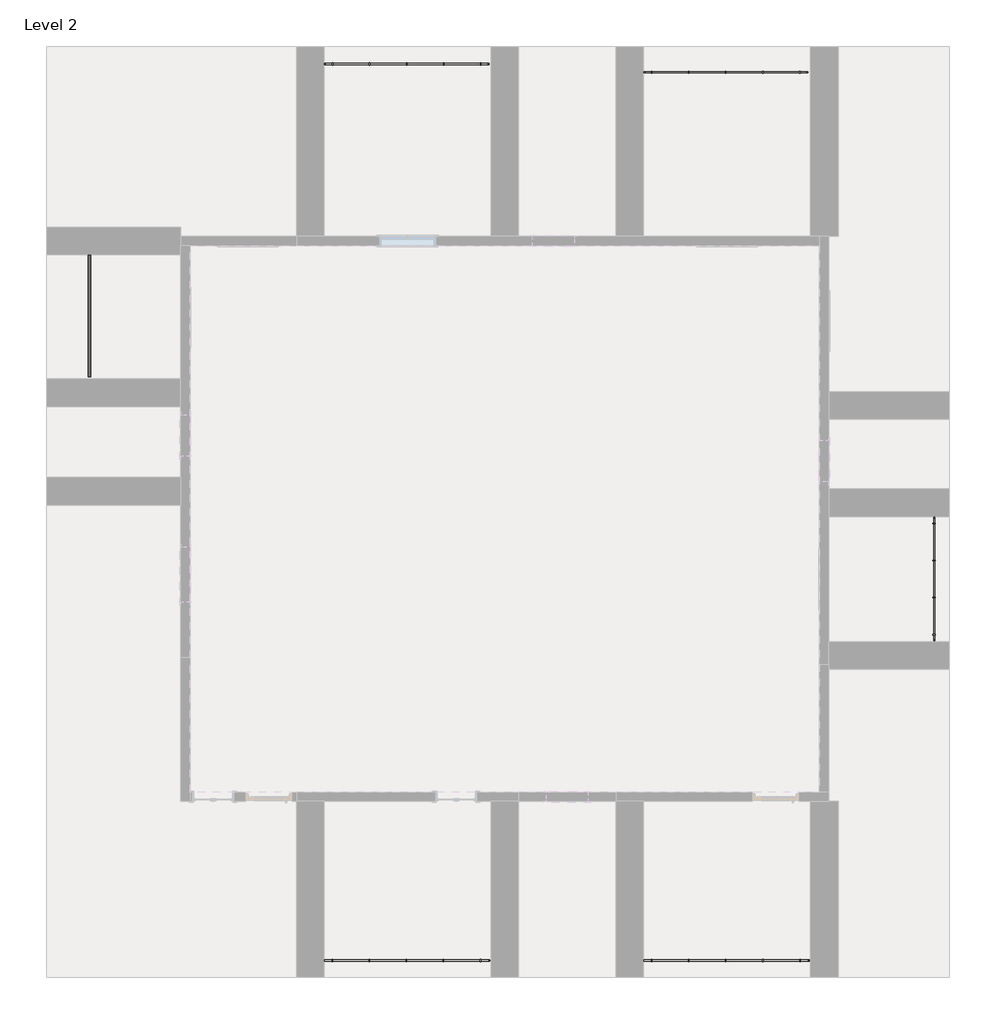
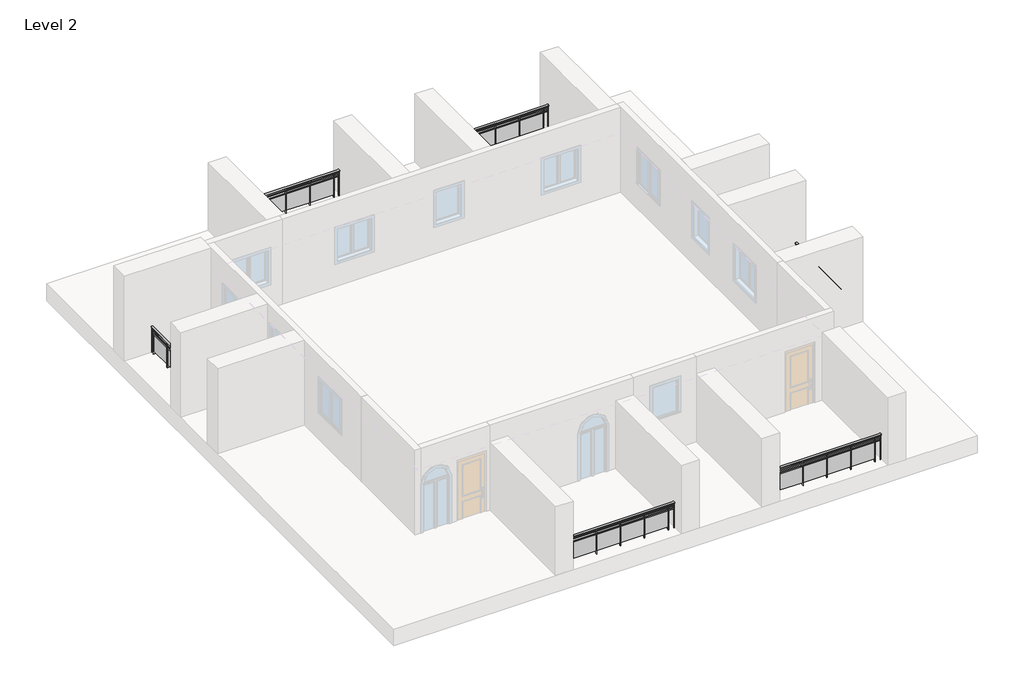
# One storey, part 2 of 2: 6 railings.
"""IFC4 building model written with IfcOpenShell, lengths in millimetres."""

from ifc_helpers import new_model, si_unit, point, frame, origin, place, context, project, spatial, polyline, ellipse_curve, trimmed, outline, extrude, element, save
from ifc_brep_helpers import plane_surface, extruded_surface, advanced_brep

model = new_model("IFC4")

# Units and contexts
model_context = context("Model", 3, world=origin())
ifc_project = project(units=[si_unit("LENGTHUNIT", "METRE", prefix="MILLI")], contexts=[model_context])

# Site, building, storey
site = spatial("IfcSite", under=ifc_project)
building = spatial("IfcBuilding", under=site)
storey = spatial("IfcBuildingStorey", under=building, Name="Level 2", Elevation=3048.0)

# Railings
placement = place(None, origin())
element("IfcRailing", 1, ObjectType="Glass Panel - Bottom Fill", at=placement, inside=storey, context=model_context, shape_type="SolidModel", body=[
    advanced_brep(
    [(-9258.4937431, -9324.2034265, 4267.2), (-9258.4937431, -9400.4034265, 4267.2), (-5600.8937431, -9324.2034265, 4267.2), (-5600.8937431, -9400.4034265, 4267.2)],
    [
        (0, 1, ellipse_curve(frame((-9258.4937431, -9362.3034265, 4267.2), z_axis=(-1.0, 0.0, 0.0), x_axis=(0.0, -1.0, 0.0)), 38.1, 28.575)),
        (1, 0, ellipse_curve(frame((-9258.4937431, -9362.3034265, 4267.2), z_axis=(-1.0, 0.0, 0.0), x_axis=(0.0, -1.0, 0.0)), 38.1, 28.575)),
        (2, 3, ellipse_curve(frame((-5600.8937431, -9362.3034265, 4267.2), z_axis=(1.0, 0.0, 0.0), x_axis=(0.0, -1.0, 0.0)), 38.1, 28.575)),
        (3, 2, ellipse_curve(frame((-5600.8937431, -9362.3034265, 4267.2), z_axis=(1.0, 0.0, 0.0), x_axis=(0.0, -1.0, 0.0)), 38.1, 28.575)),
        (0, 2),
        (3, 1),
    ],
    [
        plane_surface(frame((-9258.4937431, -9362.3034265, 4267.2), z_axis=(-1.0, 0.0, 0.0), x_axis=(0.0, 1.0, 0.0))),
        plane_surface(frame((-5600.8937431, -9362.3034265, 4267.2), z_axis=(1.0, 0.0, 0.0), x_axis=(0.0, 1.0, 0.0))),
        extruded_surface(trimmed(ellipse_curve(frame((-5600.8937431, -9362.3034265, 4267.2), z_axis=(-1.0, 0.0, 0.0), x_axis=(0.0, -1.0, 0.0)), 38.1, 28.575), [point((-5600.8937431, -9324.2034265, 4267.2))], [point((-5600.8937431, -9400.4034265, 4267.2))], True, "CARTESIAN"), (-3657.5999999999995, 0.0, 0.0), 3657.5999999999995),
        extruded_surface(trimmed(ellipse_curve(frame((-5600.8937431, -9362.3034265, 4267.2), z_axis=(-1.0, 0.0, 0.0), x_axis=(0.0, -1.0, 0.0)), 38.1, 28.575), [point((-5600.8937431, -9400.4034265, 4267.2))], [point((-5600.8937431, -9324.2034265, 4267.2))], True, "CARTESIAN"), (-3657.5999999999995, 0.0, 0.0), 3657.5999999999995),
    ],
    [
        (0, [[1, 2]]),
        (1, [[3, 4]]),
        (2, [[-1, 5, -4, 6]]),
        (3, [[-2, -6, -3, -5]]),
    ],
),
    extrude(outline(polyline([(-9258.4937431, -9375.0034265), (-9258.4937431, -9349.6034265), (-5600.8937431, -9349.6034265), (-5600.8937431, -9375.0034265), (-9258.4937431, -9375.0034265)])), frame((0.0, 0.0, 4152.9), z_axis=(0.0, 0.0, 1.0), x_axis=(1.0, 0.0, 0.0)), (0.0, 0.0, 1.0), 25.4),
    extrude(outline(polyline([(-9258.4937431, -9375.0034265), (-9258.4937431, -9349.6034265), (-5600.8937431, -9349.6034265), (-5600.8937431, -9375.0034265), (-9258.4937431, -9375.0034265)])), frame((0.0, 0.0, 4051.3), z_axis=(0.0, 0.0, 1.0), x_axis=(1.0, 0.0, 0.0)), (0.0, 0.0, 1.0), 25.4),
    extrude(outline(polyline([(-5810.4437431, -9387.7034265), (-5810.4437431, -9336.9034265), (-5797.7437431, -9336.9034265), (-5797.7437431, -9387.7034265), (-5810.4437431, -9387.7034265)])), frame((0.0, 0.0, 3352.8), z_axis=(0.0, 0.0, 1.0), x_axis=(1.0, 0.0, 0.0)), (0.0, 0.0, 1.0), 885.6788223),
    extrude(outline(polyline([(-6616.8937431, -9355.7682695), (-5804.0937431, -9355.7682695), (-5804.0937431, -9362.1182695), (-6616.8937431, -9362.1182695), (-6616.8937431, -9355.7682695)])), frame((0.0, 0.0, 3454.4), z_axis=(0.0, 0.0, 1.0), x_axis=(1.0, 0.0, 0.0)), (0.0, 0.0, 1.0), 596.9),
    extrude(outline(polyline([(-6623.2437431, -9387.7034265), (-6623.2437431, -9336.9034265), (-6610.5437431, -9336.9034265), (-6610.5437431, -9387.7034265), (-6623.2437431, -9387.7034265)])), frame((0.0, 0.0, 3352.8), z_axis=(0.0, 0.0, 1.0), x_axis=(1.0, 0.0, 0.0)), (0.0, 0.0, 1.0), 885.6788223),
    extrude(outline(polyline([(-7429.6937431, -9355.7682695), (-6616.8937431, -9355.7682695), (-6616.8937431, -9362.1182695), (-7429.6937431, -9362.1182695), (-7429.6937431, -9355.7682695)])), frame((0.0, 0.0, 3454.4), z_axis=(0.0, 0.0, 1.0), x_axis=(1.0, 0.0, 0.0)), (0.0, 0.0, 1.0), 596.9),
    extrude(outline(polyline([(-7436.0437431, -9387.7034265), (-7436.0437431, -9336.9034265), (-7423.3437431, -9336.9034265), (-7423.3437431, -9387.7034265), (-7436.0437431, -9387.7034265)])), frame((0.0, 0.0, 3352.8), z_axis=(0.0, 0.0, 1.0), x_axis=(1.0, 0.0, 0.0)), (0.0, 0.0, 1.0), 885.6788223),
    extrude(outline(polyline([(-8242.4937431, -9355.7682695), (-7429.6937431, -9355.7682695), (-7429.6937431, -9362.1182695), (-8242.4937431, -9362.1182695), (-8242.4937431, -9355.7682695)])), frame((0.0, 0.0, 3454.4), z_axis=(0.0, 0.0, 1.0), x_axis=(1.0, 0.0, 0.0)), (0.0, 0.0, 1.0), 596.9),
    extrude(outline(polyline([(-8248.8437431, -9387.7034265), (-8248.8437431, -9336.9034265), (-8236.1437431, -9336.9034265), (-8236.1437431, -9387.7034265), (-8248.8437431, -9387.7034265)])), frame((0.0, 0.0, 3352.8), z_axis=(0.0, 0.0, 1.0), x_axis=(1.0, 0.0, 0.0)), (0.0, 0.0, 1.0), 885.6788223),
    extrude(outline(polyline([(-9055.2937431, -9355.7682695), (-8242.4937431, -9355.7682695), (-8242.4937431, -9362.1182695), (-9055.2937431, -9362.1182695), (-9055.2937431, -9355.7682695)])), frame((0.0, 0.0, 3454.4), z_axis=(0.0, 0.0, 1.0), x_axis=(1.0, 0.0, 0.0)), (0.0, 0.0, 1.0), 596.9),
    extrude(outline(polyline([(-9061.6437431, -9387.7034265), (-9061.6437431, -9336.9034265), (-9048.9437431, -9336.9034265), (-9048.9437431, -9387.7034265), (-9061.6437431, -9387.7034265)])), frame((0.0, 0.0, 3352.8), z_axis=(0.0, 0.0, 1.0), x_axis=(1.0, 0.0, 0.0)), (0.0, 0.0, 1.0), 885.6788223),
    extrude(outline(polyline([(-5613.5937431, -9371.8284265), (-5613.5937431, -9352.7784265), (-5594.5437431, -9352.7784265), (-5594.5437431, -9371.8284265), (-5613.5937431, -9371.8284265)])), frame((0.0, 0.0, 3352.8), z_axis=(0.0, 0.0, 1.0), x_axis=(1.0, 0.0, 0.0)), (0.0, 0.0, 1.0), 885.6788223),
    extrude(outline(polyline([(-9264.8437431, -9371.8284265), (-9264.8437431, -9352.7784265), (-9245.7937431, -9352.7784265), (-9245.7937431, -9371.8284265), (-9264.8437431, -9371.8284265)])), frame((0.0, 0.0, 3352.8), z_axis=(0.0, 0.0, 1.0), x_axis=(1.0, 0.0, 0.0)), (0.0, 0.0, 1.0), 885.6788223),
])
element("IfcRailing", 2, ObjectType="Glass Panel - Bottom Fill", at=placement, inside=storey, context=model_context, shape_type="SolidModel", body=[
    advanced_brep(
    [(-2248.0325613, -9324.2034265, 4262.1393423), (-2248.0325613, -9400.4034265, 4262.1393423), (1409.5674387, -9324.2034265, 4262.1393423), (1409.5674387, -9400.4034265, 4262.1393423)],
    [
        (0, 1, ellipse_curve(frame((-2248.0325613, -9362.3034265, 4262.1393423), z_axis=(-1.0, 0.0, 0.0), x_axis=(0.0, -1.0, 0.0)), 38.1, 28.575)),
        (1, 0, ellipse_curve(frame((-2248.0325613, -9362.3034265, 4262.1393423), z_axis=(-1.0, 0.0, 0.0), x_axis=(0.0, -1.0, 0.0)), 38.1, 28.575)),
        (2, 3, ellipse_curve(frame((1409.5674387, -9362.3034265, 4262.1393423), z_axis=(1.0, 0.0, 0.0), x_axis=(0.0, -1.0, 0.0)), 38.1, 28.575)),
        (3, 2, ellipse_curve(frame((1409.5674387, -9362.3034265, 4262.1393423), z_axis=(1.0, 0.0, 0.0), x_axis=(0.0, -1.0, 0.0)), 38.1, 28.575)),
        (0, 2),
        (3, 1),
    ],
    [
        plane_surface(frame((-2248.0325613, -9362.3034265, 4262.1393423), z_axis=(-1.0, 0.0, 0.0), x_axis=(0.0, 1.0, 0.0))),
        plane_surface(frame((1409.5674387, -9362.3034265, 4262.1393423), z_axis=(1.0, 0.0, 0.0), x_axis=(0.0, 1.0, 0.0))),
        extruded_surface(trimmed(ellipse_curve(frame((1409.5674387, -9362.3034265, 4262.1393423), z_axis=(-1.0, 0.0, 0.0), x_axis=(0.0, -1.0, 0.0)), 38.1, 28.575), [point((1409.5674387, -9324.2034265, 4262.1393423))], [point((1409.5674387, -9400.4034265, 4262.1393423))], True, "CARTESIAN"), (-3657.6, 0.0, 0.0), 3657.6),
        extruded_surface(trimmed(ellipse_curve(frame((1409.5674387, -9362.3034265, 4262.1393423), z_axis=(-1.0, 0.0, 0.0), x_axis=(0.0, -1.0, 0.0)), 38.1, 28.575), [point((1409.5674387, -9400.4034265, 4262.1393423))], [point((1409.5674387, -9324.2034265, 4262.1393423))], True, "CARTESIAN"), (-3657.6, 0.0, 0.0), 3657.6),
    ],
    [
        (0, [[1, 2]]),
        (1, [[3, 4]]),
        (2, [[-1, 5, -4, 6]]),
        (3, [[-2, -6, -3, -5]]),
    ],
),
    extrude(outline(polyline([(-2248.0325613, -9375.0034265), (-2248.0325613, -9349.6034265), (1409.5674387, -9349.6034265), (1409.5674387, -9375.0034265), (-2248.0325613, -9375.0034265)])), frame((0.0, 0.0, 4147.8393423), z_axis=(0.0, 0.0, 1.0), x_axis=(1.0, 0.0, 0.0)), (0.0, 0.0, 1.0), 25.4),
    extrude(outline(polyline([(-2248.0325613, -9375.0034265), (-2248.0325613, -9349.6034265), (1409.5674387, -9349.6034265), (1409.5674387, -9375.0034265), (-2248.0325613, -9375.0034265)])), frame((0.0, 0.0, 4046.2393423), z_axis=(0.0, 0.0, 1.0), x_axis=(1.0, 0.0, 0.0)), (0.0, 0.0, 1.0), 25.4),
    extrude(outline(polyline([(1200.0174387, -9387.7034265), (1200.0174387, -9336.9034265), (1212.7174387, -9336.9034265), (1212.7174387, -9387.7034265), (1200.0174387, -9387.7034265)])), frame((0.0, 0.0, 3347.7393423), z_axis=(0.0, 0.0, 1.0), x_axis=(1.0, 0.0, 0.0)), (0.0, 0.0, 1.0), 885.6788223),
    extrude(outline(polyline([(393.5674387, -9355.7682695), (1206.3674387, -9355.7682695), (1206.3674387, -9362.1182695), (393.5674387, -9362.1182695), (393.5674387, -9355.7682695)])), frame((0.0, 0.0, 3449.3393423), z_axis=(0.0, 0.0, 1.0), x_axis=(1.0, 0.0, 0.0)), (0.0, 0.0, 1.0), 596.9),
    extrude(outline(polyline([(387.2174387, -9387.7034265), (387.2174387, -9336.9034265), (399.9174387, -9336.9034265), (399.9174387, -9387.7034265), (387.2174387, -9387.7034265)])), frame((0.0, 0.0, 3347.7393423), z_axis=(0.0, 0.0, 1.0), x_axis=(1.0, 0.0, 0.0)), (0.0, 0.0, 1.0), 885.6788223),
    extrude(outline(polyline([(-419.2325613, -9355.7682695), (393.5674387, -9355.7682695), (393.5674387, -9362.1182695), (-419.2325613, -9362.1182695), (-419.2325613, -9355.7682695)])), frame((0.0, 0.0, 3449.3393423), z_axis=(0.0, 0.0, 1.0), x_axis=(1.0, 0.0, 0.0)), (0.0, 0.0, 1.0), 596.9),
    extrude(outline(polyline([(-425.5825613, -9387.7034265), (-425.5825613, -9336.9034265), (-412.8825613, -9336.9034265), (-412.8825613, -9387.7034265), (-425.5825613, -9387.7034265)])), frame((0.0, 0.0, 3347.7393423), z_axis=(0.0, 0.0, 1.0), x_axis=(1.0, 0.0, 0.0)), (0.0, 0.0, 1.0), 885.6788223),
    extrude(outline(polyline([(-1232.0325613, -9355.7682695), (-419.2325613, -9355.7682695), (-419.2325613, -9362.1182695), (-1232.0325613, -9362.1182695), (-1232.0325613, -9355.7682695)])), frame((0.0, 0.0, 3449.3393423), z_axis=(0.0, 0.0, 1.0), x_axis=(1.0, 0.0, 0.0)), (0.0, 0.0, 1.0), 596.9),
    extrude(outline(polyline([(-1238.3825613, -9387.7034265), (-1238.3825613, -9336.9034265), (-1225.6825613, -9336.9034265), (-1225.6825613, -9387.7034265), (-1238.3825613, -9387.7034265)])), frame((0.0, 0.0, 3347.7393423), z_axis=(0.0, 0.0, 1.0), x_axis=(1.0, 0.0, 0.0)), (0.0, 0.0, 1.0), 885.6788223),
    extrude(outline(polyline([(-2044.8325613, -9355.7682695), (-1232.0325613, -9355.7682695), (-1232.0325613, -9362.1182695), (-2044.8325613, -9362.1182695), (-2044.8325613, -9355.7682695)])), frame((0.0, 0.0, 3449.3393423), z_axis=(0.0, 0.0, 1.0), x_axis=(1.0, 0.0, 0.0)), (0.0, 0.0, 1.0), 596.9),
    extrude(outline(polyline([(-2051.1825613, -9387.7034265), (-2051.1825613, -9336.9034265), (-2038.4825613, -9336.9034265), (-2038.4825613, -9387.7034265), (-2051.1825613, -9387.7034265)])), frame((0.0, 0.0, 3347.7393423), z_axis=(0.0, 0.0, 1.0), x_axis=(1.0, 0.0, 0.0)), (0.0, 0.0, 1.0), 885.6788223),
    extrude(outline(polyline([(1396.8674387, -9371.8284265), (1396.8674387, -9352.7784265), (1415.9174387, -9352.7784265), (1415.9174387, -9371.8284265), (1396.8674387, -9371.8284265)])), frame((0.0, 0.0, 3347.7393423), z_axis=(0.0, 0.0, 1.0), x_axis=(1.0, 0.0, 0.0)), (0.0, 0.0, 1.0), 885.6788223),
    extrude(outline(polyline([(-2254.3825613, -9371.8284265), (-2254.3825613, -9352.7784265), (-2235.3325613, -9352.7784265), (-2235.3325613, -9371.8284265), (-2254.3825613, -9371.8284265)])), frame((0.0, 0.0, 3347.7393423), z_axis=(0.0, 0.0, 1.0), x_axis=(1.0, 0.0, 0.0)), (0.0, 0.0, 1.0), 885.6788223),
])
element("IfcRailing", 3, ObjectType="Glass Panel - Bottom Fill", at=placement, inside=storey, context=model_context, shape_type="SolidModel", body=[
    advanced_brep(
    [(-14351.1937431, 6115.813611, 4267.2), (-14427.3937431, 6115.813611, 4267.2), (-14351.1937431, 3448.813611, 4267.2), (-14427.3937431, 3448.813611, 4267.2)],
    [
        (0, 1, ellipse_curve(frame((-14389.2937431, 6115.813611, 4267.2), z_axis=(0.0, 1.0, 0.0), x_axis=(-1.0, 0.0, 0.0)), 38.1, 28.575)),
        (1, 0, ellipse_curve(frame((-14389.2937431, 6115.813611, 4267.2), z_axis=(0.0, 1.0, 0.0), x_axis=(-1.0, 0.0, 0.0)), 38.1, 28.575)),
        (2, 3, ellipse_curve(frame((-14389.2937431, 3448.813611, 4267.2), z_axis=(0.0, -1.0, 0.0), x_axis=(-1.0, 0.0, 0.0)), 38.1, 28.575)),
        (3, 2, ellipse_curve(frame((-14389.2937431, 3448.813611, 4267.2), z_axis=(0.0, -1.0, 0.0), x_axis=(-1.0, 0.0, 0.0)), 38.1, 28.575)),
        (0, 2),
        (3, 1),
    ],
    [
        plane_surface(frame((-14389.2937431, 6115.813611, 4267.2), z_axis=(0.0, 1.0, 0.0), x_axis=(0.0, 0.0, -1.0))),
        plane_surface(frame((-14389.2937431, 3448.813611, 4267.2), z_axis=(0.0, -1.0, 0.0), x_axis=(0.0, 0.0, -1.0))),
        extruded_surface(trimmed(ellipse_curve(frame((-14389.2937431, 3448.813611, 4267.2), z_axis=(0.0, 1.0, 0.0), x_axis=(-1.0, 0.0, 0.0)), 38.1, 28.575), [point((-14351.1937431, 3448.813611, 4267.2))], [point((-14427.3937431, 3448.813611, 4267.2))], True, "CARTESIAN"), (0.0, 2666.9999999999995, 0.0), 2666.9999999999995),
        extruded_surface(trimmed(ellipse_curve(frame((-14389.2937431, 3448.813611, 4267.2), z_axis=(0.0, 1.0, 0.0), x_axis=(-1.0, 0.0, 0.0)), 38.1, 28.575), [point((-14427.3937431, 3448.813611, 4267.2))], [point((-14351.1937431, 3448.813611, 4267.2))], True, "CARTESIAN"), (0.0, 2666.9999999999995, 0.0), 2666.9999999999995),
    ],
    [
        (0, [[1, 2]]),
        (1, [[3, 4]]),
        (2, [[-1, 5, -4, 6]]),
        (3, [[-2, -6, -3, -5]]),
    ],
),
    extrude(outline(polyline([(-14401.9937431, 6115.813611), (-14376.5937431, 6115.813611), (-14376.5937431, 3448.813611), (-14401.9937431, 3448.813611), (-14401.9937431, 6115.813611)])), frame((0.0, 0.0, 4152.9), z_axis=(0.0, 0.0, 1.0), x_axis=(1.0, 0.0, 0.0)), (0.0, 0.0, 1.0), 25.4),
    extrude(outline(polyline([(-14401.9937431, 6115.813611), (-14376.5937431, 6115.813611), (-14376.5937431, 3448.813611), (-14401.9937431, 3448.813611), (-14401.9937431, 6115.813611)])), frame((0.0, 0.0, 4051.3), z_axis=(0.0, 0.0, 1.0), x_axis=(1.0, 0.0, 0.0)), (0.0, 0.0, 1.0), 25.4),
    extrude(outline(polyline([(-14414.6937431, 3569.463611), (-14363.8937431, 3569.463611), (-14363.8937431, 3556.763611), (-14414.6937431, 3556.763611), (-14414.6937431, 3569.463611)])), frame((0.0, 0.0, 3352.8), z_axis=(0.0, 0.0, 1.0), x_axis=(1.0, 0.0, 0.0)), (0.0, 0.0, 1.0), 885.6788223),
    extrude(outline(polyline([(-14382.7585861, 4375.913611), (-14382.7585861, 3563.113611), (-14389.1085861, 3563.113611), (-14389.1085861, 4375.913611), (-14382.7585861, 4375.913611)])), frame((0.0, 0.0, 3454.4), z_axis=(0.0, 0.0, 1.0), x_axis=(1.0, 0.0, 0.0)), (0.0, 0.0, 1.0), 596.9),
    extrude(outline(polyline([(-14414.6937431, 4382.263611), (-14363.8937431, 4382.263611), (-14363.8937431, 4369.563611), (-14414.6937431, 4369.563611), (-14414.6937431, 4382.263611)])), frame((0.0, 0.0, 3352.8), z_axis=(0.0, 0.0, 1.0), x_axis=(1.0, 0.0, 0.0)), (0.0, 0.0, 1.0), 885.6788223),
    extrude(outline(polyline([(-14382.7585861, 5188.713611), (-14382.7585861, 4375.913611), (-14389.1085861, 4375.913611), (-14389.1085861, 5188.713611), (-14382.7585861, 5188.713611)])), frame((0.0, 0.0, 3454.4), z_axis=(0.0, 0.0, 1.0), x_axis=(1.0, 0.0, 0.0)), (0.0, 0.0, 1.0), 596.9),
    extrude(outline(polyline([(-14414.6937431, 5195.063611), (-14363.8937431, 5195.063611), (-14363.8937431, 5182.363611), (-14414.6937431, 5182.363611), (-14414.6937431, 5195.063611)])), frame((0.0, 0.0, 3352.8), z_axis=(0.0, 0.0, 1.0), x_axis=(1.0, 0.0, 0.0)), (0.0, 0.0, 1.0), 885.6788223),
    extrude(outline(polyline([(-14382.7585861, 6001.513611), (-14382.7585861, 5188.713611), (-14389.1085861, 5188.713611), (-14389.1085861, 6001.513611), (-14382.7585861, 6001.513611)])), frame((0.0, 0.0, 3454.4), z_axis=(0.0, 0.0, 1.0), x_axis=(1.0, 0.0, 0.0)), (0.0, 0.0, 1.0), 596.9),
    extrude(outline(polyline([(-14414.6937431, 6007.863611), (-14363.8937431, 6007.863611), (-14363.8937431, 5995.163611), (-14414.6937431, 5995.163611), (-14414.6937431, 6007.863611)])), frame((0.0, 0.0, 3352.8), z_axis=(0.0, 0.0, 1.0), x_axis=(1.0, 0.0, 0.0)), (0.0, 0.0, 1.0), 885.6788223),
    extrude(outline(polyline([(-14398.8187431, 3461.513611), (-14379.7687431, 3461.513611), (-14379.7687431, 3442.463611), (-14398.8187431, 3442.463611), (-14398.8187431, 3461.513611)])), frame((0.0, 0.0, 3352.8), z_axis=(0.0, 0.0, 1.0), x_axis=(1.0, 0.0, 0.0)), (0.0, 0.0, 1.0), 885.6788223),
    extrude(outline(polyline([(-14398.8187431, 6122.163611), (-14379.7687431, 6122.163611), (-14379.7687431, 6103.113611), (-14398.8187431, 6103.113611), (-14398.8187431, 6122.163611)])), frame((0.0, 0.0, 3352.8), z_axis=(0.0, 0.0, 1.0), x_axis=(1.0, 0.0, 0.0)), (0.0, 0.0, 1.0), 885.6788223),
])
element("IfcRailing", 4, ObjectType="Glass Panel - Bottom Fill", at=placement, inside=storey, context=model_context, shape_type="SolidModel", body=[
    advanced_brep(
    [(-9229.0758442, 10344.5205237, 4267.2), (-9229.0758442, 10268.3205237, 4267.2), (-5622.2758442, 10344.5205237, 4267.2), (-5622.2758442, 10268.3205237, 4267.2)],
    [
        (0, 1, ellipse_curve(frame((-9229.0758442, 10306.4205237, 4267.2), z_axis=(-1.0, 0.0, 0.0), x_axis=(0.0, -1.0, 0.0)), 38.1, 28.575)),
        (1, 0, ellipse_curve(frame((-9229.0758442, 10306.4205237, 4267.2), z_axis=(-1.0, 0.0, 0.0), x_axis=(0.0, -1.0, 0.0)), 38.1, 28.575)),
        (2, 3, ellipse_curve(frame((-5622.2758442, 10306.4205237, 4267.2), z_axis=(1.0, 0.0, 0.0), x_axis=(0.0, -1.0, 0.0)), 38.1, 28.575)),
        (3, 2, ellipse_curve(frame((-5622.2758442, 10306.4205237, 4267.2), z_axis=(1.0, 0.0, 0.0), x_axis=(0.0, -1.0, 0.0)), 38.1, 28.575)),
        (0, 2),
        (3, 1),
    ],
    [
        plane_surface(frame((-9229.0758442, 10306.4205237, 4267.2), z_axis=(-1.0, 0.0, 0.0), x_axis=(0.0, 1.0, 0.0))),
        plane_surface(frame((-5622.2758442, 10306.4205237, 4267.2), z_axis=(1.0, 0.0, 0.0), x_axis=(0.0, 1.0, 0.0))),
        extruded_surface(trimmed(ellipse_curve(frame((-5622.2758442, 10306.4205237, 4267.2), z_axis=(-1.0, 0.0, 0.0), x_axis=(0.0, -1.0, 0.0)), 38.1, 28.575), [point((-5622.2758442, 10344.5205237, 4267.2))], [point((-5622.2758442, 10268.3205237, 4267.2))], True, "CARTESIAN"), (-3606.8, 0.0, 0.0), 3606.8),
        extruded_surface(trimmed(ellipse_curve(frame((-5622.2758442, 10306.4205237, 4267.2), z_axis=(-1.0, 0.0, 0.0), x_axis=(0.0, -1.0, 0.0)), 38.1, 28.575), [point((-5622.2758442, 10268.3205237, 4267.2))], [point((-5622.2758442, 10344.5205237, 4267.2))], True, "CARTESIAN"), (-3606.8, 0.0, 0.0), 3606.8),
    ],
    [
        (0, [[1, 2]]),
        (1, [[3, 4]]),
        (2, [[-1, 5, -4, 6]]),
        (3, [[-2, -6, -3, -5]]),
    ],
),
    extrude(outline(polyline([(-9229.0758442, 10293.7205237), (-9229.0758442, 10319.1205237), (-5622.2758442, 10319.1205237), (-5622.2758442, 10293.7205237), (-9229.0758442, 10293.7205237)])), frame((0.0, 0.0, 4152.9), z_axis=(0.0, 0.0, 1.0), x_axis=(1.0, 0.0, 0.0)), (0.0, 0.0, 1.0), 25.4),
    extrude(outline(polyline([(-9229.0758442, 10293.7205237), (-9229.0758442, 10319.1205237), (-5622.2758442, 10319.1205237), (-5622.2758442, 10293.7205237), (-9229.0758442, 10293.7205237)])), frame((0.0, 0.0, 4051.3), z_axis=(0.0, 0.0, 1.0), x_axis=(1.0, 0.0, 0.0)), (0.0, 0.0, 1.0), 25.4),
    extrude(outline(polyline([(-5806.4258442, 10281.0205237), (-5806.4258442, 10331.8205237), (-5793.7258442, 10331.8205237), (-5793.7258442, 10281.0205237), (-5806.4258442, 10281.0205237)])), frame((0.0, 0.0, 3352.8), z_axis=(0.0, 0.0, 1.0), x_axis=(1.0, 0.0, 0.0)), (0.0, 0.0, 1.0), 885.6788223),
    extrude(outline(polyline([(-6612.8758442, 10312.9556807), (-5800.0758442, 10312.9556807), (-5800.0758442, 10306.6056807), (-6612.8758442, 10306.6056807), (-6612.8758442, 10312.9556807)])), frame((0.0, 0.0, 3454.4), z_axis=(0.0, 0.0, 1.0), x_axis=(1.0, 0.0, 0.0)), (0.0, 0.0, 1.0), 596.9),
    extrude(outline(polyline([(-6619.2258442, 10281.0205237), (-6619.2258442, 10331.8205237), (-6606.5258442, 10331.8205237), (-6606.5258442, 10281.0205237), (-6619.2258442, 10281.0205237)])), frame((0.0, 0.0, 3352.8), z_axis=(0.0, 0.0, 1.0), x_axis=(1.0, 0.0, 0.0)), (0.0, 0.0, 1.0), 885.6788223),
    extrude(outline(polyline([(-7425.6758442, 10312.9556807), (-6612.8758442, 10312.9556807), (-6612.8758442, 10306.6056807), (-7425.6758442, 10306.6056807), (-7425.6758442, 10312.9556807)])), frame((0.0, 0.0, 3454.4), z_axis=(0.0, 0.0, 1.0), x_axis=(1.0, 0.0, 0.0)), (0.0, 0.0, 1.0), 596.9),
    extrude(outline(polyline([(-7432.0258442, 10281.0205237), (-7432.0258442, 10331.8205237), (-7419.3258442, 10331.8205237), (-7419.3258442, 10281.0205237), (-7432.0258442, 10281.0205237)])), frame((0.0, 0.0, 3352.8), z_axis=(0.0, 0.0, 1.0), x_axis=(1.0, 0.0, 0.0)), (0.0, 0.0, 1.0), 885.6788223),
    extrude(outline(polyline([(-8238.4758442, 10312.9556807), (-7425.6758442, 10312.9556807), (-7425.6758442, 10306.6056807), (-8238.4758442, 10306.6056807), (-8238.4758442, 10312.9556807)])), frame((0.0, 0.0, 3454.4), z_axis=(0.0, 0.0, 1.0), x_axis=(1.0, 0.0, 0.0)), (0.0, 0.0, 1.0), 596.9),
    extrude(outline(polyline([(-8244.8258442, 10281.0205237), (-8244.8258442, 10331.8205237), (-8232.1258442, 10331.8205237), (-8232.1258442, 10281.0205237), (-8244.8258442, 10281.0205237)])), frame((0.0, 0.0, 3352.8), z_axis=(0.0, 0.0, 1.0), x_axis=(1.0, 0.0, 0.0)), (0.0, 0.0, 1.0), 885.6788223),
    extrude(outline(polyline([(-9051.2758442, 10312.9556807), (-8238.4758442, 10312.9556807), (-8238.4758442, 10306.6056807), (-9051.2758442, 10306.6056807), (-9051.2758442, 10312.9556807)])), frame((0.0, 0.0, 3454.4), z_axis=(0.0, 0.0, 1.0), x_axis=(1.0, 0.0, 0.0)), (0.0, 0.0, 1.0), 596.9),
    extrude(outline(polyline([(-9057.6258442, 10281.0205237), (-9057.6258442, 10331.8205237), (-9044.9258442, 10331.8205237), (-9044.9258442, 10281.0205237), (-9057.6258442, 10281.0205237)])), frame((0.0, 0.0, 3352.8), z_axis=(0.0, 0.0, 1.0), x_axis=(1.0, 0.0, 0.0)), (0.0, 0.0, 1.0), 885.6788223),
    extrude(outline(polyline([(-5634.9758442, 10296.8955237), (-5634.9758442, 10315.9455237), (-5615.9258442, 10315.9455237), (-5615.9258442, 10296.8955237), (-5634.9758442, 10296.8955237)])), frame((0.0, 0.0, 3352.8), z_axis=(0.0, 0.0, 1.0), x_axis=(1.0, 0.0, 0.0)), (0.0, 0.0, 1.0), 885.6788223),
    extrude(outline(polyline([(-9235.4258442, 10296.8955237), (-9235.4258442, 10315.9455237), (-9216.3758442, 10315.9455237), (-9216.3758442, 10296.8955237), (-9235.4258442, 10296.8955237)])), frame((0.0, 0.0, 3352.8), z_axis=(0.0, 0.0, 1.0), x_axis=(1.0, 0.0, 0.0)), (0.0, 0.0, 1.0), 885.6788223),
])
element("IfcRailing", 5, ObjectType="Glass Panel - Bottom Fill", at=placement, inside=storey, context=model_context, shape_type="SolidModel", body=[
    advanced_brep(
    [(-2210.3891352, 10161.3373193, 4267.2), (-2210.3891352, 10085.1373193, 4267.2), (1371.0108648, 10161.3373193, 4267.2), (1371.0108648, 10085.1373193, 4267.2)],
    [
        (0, 1, ellipse_curve(frame((-2210.3891352, 10123.2373193, 4267.2), z_axis=(-1.0, 0.0, 0.0), x_axis=(0.0, -1.0, 0.0)), 38.1, 28.575)),
        (1, 0, ellipse_curve(frame((-2210.3891352, 10123.2373193, 4267.2), z_axis=(-1.0, 0.0, 0.0), x_axis=(0.0, -1.0, 0.0)), 38.1, 28.575)),
        (2, 3, ellipse_curve(frame((1371.0108648, 10123.2373193, 4267.2), z_axis=(1.0, 0.0, 0.0), x_axis=(0.0, -1.0, 0.0)), 38.1, 28.575)),
        (3, 2, ellipse_curve(frame((1371.0108648, 10123.2373193, 4267.2), z_axis=(1.0, 0.0, 0.0), x_axis=(0.0, -1.0, 0.0)), 38.1, 28.575)),
        (0, 2),
        (3, 1),
    ],
    [
        plane_surface(frame((-2210.3891352, 10123.2373193, 4267.2), z_axis=(-1.0, 0.0, 0.0), x_axis=(0.0, 1.0, 0.0))),
        plane_surface(frame((1371.0108648, 10123.2373193, 4267.2), z_axis=(1.0, 0.0, 0.0), x_axis=(0.0, 1.0, 0.0))),
        extruded_surface(trimmed(ellipse_curve(frame((1371.0108648, 10123.2373193, 4267.2), z_axis=(-1.0, 0.0, 0.0), x_axis=(0.0, -1.0, 0.0)), 38.1, 28.575), [point((1371.0108648, 10161.3373193, 4267.2))], [point((1371.0108648, 10085.1373193, 4267.2))], True, "CARTESIAN"), (-3581.4, 0.0, 0.0), 3581.4),
        extruded_surface(trimmed(ellipse_curve(frame((1371.0108648, 10123.2373193, 4267.2), z_axis=(-1.0, 0.0, 0.0), x_axis=(0.0, -1.0, 0.0)), 38.1, 28.575), [point((1371.0108648, 10085.1373193, 4267.2))], [point((1371.0108648, 10161.3373193, 4267.2))], True, "CARTESIAN"), (-3581.4, 0.0, 0.0), 3581.4),
    ],
    [
        (0, [[1, 2]]),
        (1, [[3, 4]]),
        (2, [[-1, 5, -4, 6]]),
        (3, [[-2, -6, -3, -5]]),
    ],
),
    extrude(outline(polyline([(-2210.3891352, 10110.5373193), (-2210.3891352, 10135.9373193), (1371.0108648, 10135.9373193), (1371.0108648, 10110.5373193), (-2210.3891352, 10110.5373193)])), frame((0.0, 0.0, 4152.9), z_axis=(0.0, 0.0, 1.0), x_axis=(1.0, 0.0, 0.0)), (0.0, 0.0, 1.0), 25.4),
    extrude(outline(polyline([(-2210.3891352, 10110.5373193), (-2210.3891352, 10135.9373193), (1371.0108648, 10135.9373193), (1371.0108648, 10110.5373193), (-2210.3891352, 10110.5373193)])), frame((0.0, 0.0, 4051.3), z_axis=(0.0, 0.0, 1.0), x_axis=(1.0, 0.0, 0.0)), (0.0, 0.0, 1.0), 25.4),
    extrude(outline(polyline([(1199.5608648, 10097.8373193), (1199.5608648, 10148.6373193), (1212.2608648, 10148.6373193), (1212.2608648, 10097.8373193), (1199.5608648, 10097.8373193)])), frame((0.0, 0.0, 3352.8), z_axis=(0.0, 0.0, 1.0), x_axis=(1.0, 0.0, 0.0)), (0.0, 0.0, 1.0), 885.6788223),
    extrude(outline(polyline([(393.1108648, 10129.7724763), (1205.9108648, 10129.7724763), (1205.9108648, 10123.4224763), (393.1108648, 10123.4224763), (393.1108648, 10129.7724763)])), frame((0.0, 0.0, 3454.4), z_axis=(0.0, 0.0, 1.0), x_axis=(1.0, 0.0, 0.0)), (0.0, 0.0, 1.0), 596.9),
    extrude(outline(polyline([(386.7608648, 10097.8373193), (386.7608648, 10148.6373193), (399.4608648, 10148.6373193), (399.4608648, 10097.8373193), (386.7608648, 10097.8373193)])), frame((0.0, 0.0, 3352.8), z_axis=(0.0, 0.0, 1.0), x_axis=(1.0, 0.0, 0.0)), (0.0, 0.0, 1.0), 885.6788223),
    extrude(outline(polyline([(-419.6891352, 10129.7724763), (393.1108648, 10129.7724763), (393.1108648, 10123.4224763), (-419.6891352, 10123.4224763), (-419.6891352, 10129.7724763)])), frame((0.0, 0.0, 3454.4), z_axis=(0.0, 0.0, 1.0), x_axis=(1.0, 0.0, 0.0)), (0.0, 0.0, 1.0), 596.9),
    extrude(outline(polyline([(-426.0391352, 10097.8373193), (-426.0391352, 10148.6373193), (-413.3391352, 10148.6373193), (-413.3391352, 10097.8373193), (-426.0391352, 10097.8373193)])), frame((0.0, 0.0, 3352.8), z_axis=(0.0, 0.0, 1.0), x_axis=(1.0, 0.0, 0.0)), (0.0, 0.0, 1.0), 885.6788223),
    extrude(outline(polyline([(-1232.4891352, 10129.7724763), (-419.6891352, 10129.7724763), (-419.6891352, 10123.4224763), (-1232.4891352, 10123.4224763), (-1232.4891352, 10129.7724763)])), frame((0.0, 0.0, 3454.4), z_axis=(0.0, 0.0, 1.0), x_axis=(1.0, 0.0, 0.0)), (0.0, 0.0, 1.0), 596.9),
    extrude(outline(polyline([(-1238.8391352, 10097.8373193), (-1238.8391352, 10148.6373193), (-1226.1391352, 10148.6373193), (-1226.1391352, 10097.8373193), (-1238.8391352, 10097.8373193)])), frame((0.0, 0.0, 3352.8), z_axis=(0.0, 0.0, 1.0), x_axis=(1.0, 0.0, 0.0)), (0.0, 0.0, 1.0), 885.6788223),
    extrude(outline(polyline([(-2045.2891352, 10129.7724763), (-1232.4891352, 10129.7724763), (-1232.4891352, 10123.4224763), (-2045.2891352, 10123.4224763), (-2045.2891352, 10129.7724763)])), frame((0.0, 0.0, 3454.4), z_axis=(0.0, 0.0, 1.0), x_axis=(1.0, 0.0, 0.0)), (0.0, 0.0, 1.0), 596.9),
    extrude(outline(polyline([(-2051.6391352, 10097.8373193), (-2051.6391352, 10148.6373193), (-2038.9391352, 10148.6373193), (-2038.9391352, 10097.8373193), (-2051.6391352, 10097.8373193)])), frame((0.0, 0.0, 3352.8), z_axis=(0.0, 0.0, 1.0), x_axis=(1.0, 0.0, 0.0)), (0.0, 0.0, 1.0), 885.6788223),
    extrude(outline(polyline([(1358.3108648, 10113.7123193), (1358.3108648, 10132.7623193), (1377.3608648, 10132.7623193), (1377.3608648, 10113.7123193), (1358.3108648, 10113.7123193)])), frame((0.0, 0.0, 3352.8), z_axis=(0.0, 0.0, 1.0), x_axis=(1.0, 0.0, 0.0)), (0.0, 0.0, 1.0), 885.6788223),
    extrude(outline(polyline([(-2216.7391352, 10113.7123193), (-2216.7391352, 10132.7623193), (-2197.6891352, 10132.7623193), (-2197.6891352, 10113.7123193), (-2216.7391352, 10113.7123193)])), frame((0.0, 0.0, 3352.8), z_axis=(0.0, 0.0, 1.0), x_axis=(1.0, 0.0, 0.0)), (0.0, 0.0, 1.0), 885.6788223),
])
element("IfcRailing", 6, ObjectType="Glass Panel - Bottom Fill", at=placement, inside=storey, context=model_context, shape_type="SolidModel", body=[
    advanced_brep(
    [(4190.8062569, 350.013611, 4267.2), (4114.6062569, 350.013611, 4267.2), (4190.8062569, -2342.386389, 4267.2), (4114.6062569, -2342.386389, 4267.2)],
    [
        (0, 1, ellipse_curve(frame((4152.7062569, 350.013611, 4267.2), z_axis=(0.0, 1.0, 0.0), x_axis=(-1.0, 0.0, 0.0)), 38.1, 28.575)),
        (1, 0, ellipse_curve(frame((4152.7062569, 350.013611, 4267.2), z_axis=(0.0, 1.0, 0.0), x_axis=(-1.0, 0.0, 0.0)), 38.1, 28.575)),
        (2, 3, ellipse_curve(frame((4152.7062569, -2342.386389, 4267.2), z_axis=(0.0, -1.0, 0.0), x_axis=(-1.0, 0.0, 0.0)), 38.1, 28.575)),
        (3, 2, ellipse_curve(frame((4152.7062569, -2342.386389, 4267.2), z_axis=(0.0, -1.0, 0.0), x_axis=(-1.0, 0.0, 0.0)), 38.1, 28.575)),
        (0, 2),
        (3, 1),
    ],
    [
        plane_surface(frame((4152.7062569, 350.013611, 4267.2), z_axis=(0.0, 1.0, 0.0), x_axis=(0.0, 0.0, -1.0))),
        plane_surface(frame((4152.7062569, -2342.386389, 4267.2), z_axis=(0.0, -1.0, 0.0), x_axis=(0.0, 0.0, -1.0))),
        extruded_surface(trimmed(ellipse_curve(frame((4152.7062569, -2342.386389, 4267.2), z_axis=(0.0, 1.0, 0.0), x_axis=(-1.0, 0.0, 0.0)), 38.1, 28.575), [point((4190.8062569, -2342.386389, 4267.2))], [point((4114.6062569, -2342.386389, 4267.2))], True, "CARTESIAN"), (0.0, 2692.3999999999996, 0.0), 2692.3999999999996),
        extruded_surface(trimmed(ellipse_curve(frame((4152.7062569, -2342.386389, 4267.2), z_axis=(0.0, 1.0, 0.0), x_axis=(-1.0, 0.0, 0.0)), 38.1, 28.575), [point((4114.6062569, -2342.386389, 4267.2))], [point((4190.8062569, -2342.386389, 4267.2))], True, "CARTESIAN"), (0.0, 2692.3999999999996, 0.0), 2692.3999999999996),
    ],
    [
        (0, [[1, 2]]),
        (1, [[3, 4]]),
        (2, [[-1, 5, -4, 6]]),
        (3, [[-2, -6, -3, -5]]),
    ],
),
    extrude(outline(polyline([(4140.0062569, 350.013611), (4165.4062569, 350.013611), (4165.4062569, -2342.386389), (4140.0062569, -2342.386389), (4140.0062569, 350.013611)])), frame((0.0, 0.0, 4152.9), z_axis=(0.0, 0.0, 1.0), x_axis=(1.0, 0.0, 0.0)), (0.0, 0.0, 1.0), 25.4),
    extrude(outline(polyline([(4140.0062569, 350.013611), (4165.4062569, 350.013611), (4165.4062569, -2342.386389), (4140.0062569, -2342.386389), (4140.0062569, 350.013611)])), frame((0.0, 0.0, 4051.3), z_axis=(0.0, 0.0, 1.0), x_axis=(1.0, 0.0, 0.0)), (0.0, 0.0, 1.0), 25.4),
    extrude(outline(polyline([(4127.3062569, -2209.036389), (4178.1062569, -2209.036389), (4178.1062569, -2221.736389), (4127.3062569, -2221.736389), (4127.3062569, -2209.036389)])), frame((0.0, 0.0, 3352.8), z_axis=(0.0, 0.0, 1.0), x_axis=(1.0, 0.0, 0.0)), (0.0, 0.0, 1.0), 885.6788223),
    extrude(outline(polyline([(4159.2414139, -1402.586389), (4159.2414139, -2215.386389), (4152.8914139, -2215.386389), (4152.8914139, -1402.586389), (4159.2414139, -1402.586389)])), frame((0.0, 0.0, 3454.4), z_axis=(0.0, 0.0, 1.0), x_axis=(1.0, 0.0, 0.0)), (0.0, 0.0, 1.0), 596.9),
    extrude(outline(polyline([(4127.3062569, -1396.236389), (4178.1062569, -1396.236389), (4178.1062569, -1408.936389), (4127.3062569, -1408.936389), (4127.3062569, -1396.236389)])), frame((0.0, 0.0, 3352.8), z_axis=(0.0, 0.0, 1.0), x_axis=(1.0, 0.0, 0.0)), (0.0, 0.0, 1.0), 885.6788223),
    extrude(outline(polyline([(4159.2414139, -589.786389), (4159.2414139, -1402.586389), (4152.8914139, -1402.586389), (4152.8914139, -589.786389), (4159.2414139, -589.786389)])), frame((0.0, 0.0, 3454.4), z_axis=(0.0, 0.0, 1.0), x_axis=(1.0, 0.0, 0.0)), (0.0, 0.0, 1.0), 596.9),
    extrude(outline(polyline([(4127.3062569, -583.436389), (4178.1062569, -583.436389), (4178.1062569, -596.136389), (4127.3062569, -596.136389), (4127.3062569, -583.436389)])), frame((0.0, 0.0, 3352.8), z_axis=(0.0, 0.0, 1.0), x_axis=(1.0, 0.0, 0.0)), (0.0, 0.0, 1.0), 885.6788223),
    extrude(outline(polyline([(4159.2414139, 223.013611), (4159.2414139, -589.786389), (4152.8914139, -589.786389), (4152.8914139, 223.013611), (4159.2414139, 223.013611)])), frame((0.0, 0.0, 3454.4), z_axis=(0.0, 0.0, 1.0), x_axis=(1.0, 0.0, 0.0)), (0.0, 0.0, 1.0), 596.9),
    extrude(outline(polyline([(4127.3062569, 229.363611), (4178.1062569, 229.363611), (4178.1062569, 216.663611), (4127.3062569, 216.663611), (4127.3062569, 229.363611)])), frame((0.0, 0.0, 3352.8), z_axis=(0.0, 0.0, 1.0), x_axis=(1.0, 0.0, 0.0)), (0.0, 0.0, 1.0), 885.6788223),
    extrude(outline(polyline([(4143.1812569, -2329.686389), (4162.2312569, -2329.686389), (4162.2312569, -2348.736389), (4143.1812569, -2348.736389), (4143.1812569, -2329.686389)])), frame((0.0, 0.0, 3352.8), z_axis=(0.0, 0.0, 1.0), x_axis=(1.0, 0.0, 0.0)), (0.0, 0.0, 1.0), 885.6788223),
    extrude(outline(polyline([(4143.1812569, 356.363611), (4162.2312569, 356.363611), (4162.2312569, 337.313611), (4143.1812569, 337.313611), (4143.1812569, 356.363611)])), frame((0.0, 0.0, 3352.8), z_axis=(0.0, 0.0, 1.0), x_axis=(1.0, 0.0, 0.0)), (0.0, 0.0, 1.0), 885.6788223),
])

save(model, "model.ifc")

# Revit data of these elements
# Type "Glass Panel - Bottom Fill"
#   Assembly Code = "C2010400"
#   built-in parameter 1008612 = 0.0416667 (stored number, unit not read)
#   built-in parameter 1008611 = 0.0416667 (stored number, unit not read)
#   built-in parameter 1008609 = 0.333333 (stored number, unit not read)
#   built-in parameter 1008604 = 0.166667 (stored number, unit not read)
#   built-in parameter 1008603 = 0.166667 (stored number, unit not read)
#   Railing Height = 3' - 0"
#   built-in parameter 1008630 = 2
#   built-in parameter 1008610 = 2
#   built-in parameter 1008618 = Baluster - Square : 3/4"
# Elements 1, 3, 4, 5, 6 (IfcRailing, "Glass Panel - Bottom Fill")
#   built-in parameter 1008621 = 1 (stored number, unit not read)
#   Phase Created = New Construction
#   Materials on its faces: "Glass"
# Element 2 (IfcRailing, "Glass Panel - Bottom Fill")
#   built-in parameter 1008621 = 0.983397 (stored number, unit not read)
#   Phase Created = New Construction
#   Materials on its faces: "Glass"
# Materials
#   "Glass": class "Glass", colour RGB 0 128 192, transparency 0.75, Description = "Soda Lime Glass", Cost = 0
